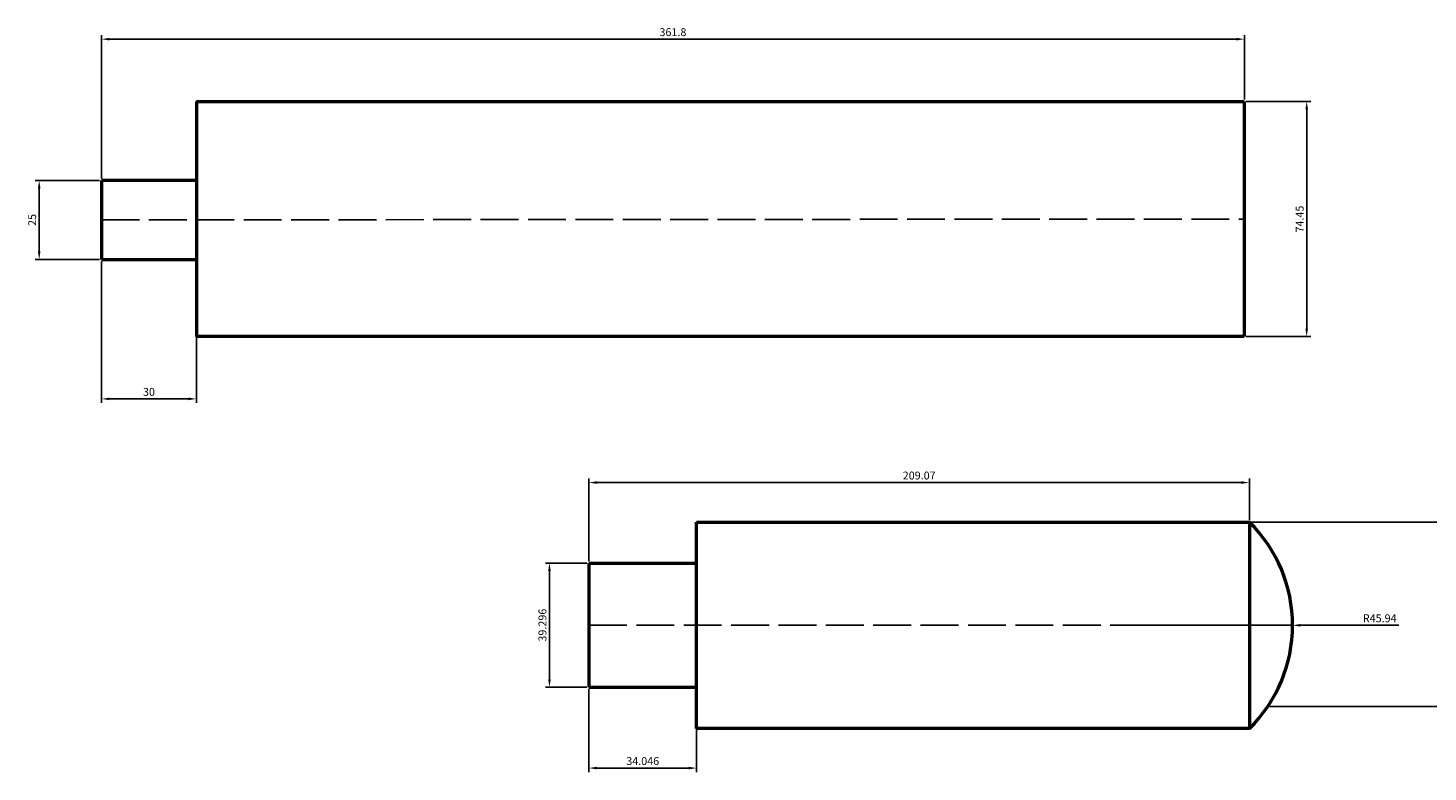
# Model space of a CAD drawing. Units: millimetres. Extents: x 921 to 2648, y 1390 to 2315.
# Tile 6 of 10: x 1762 to 2205, y 1390 to 1625. Entities that reach past the tile are written whole.
import ezdxf

# ---------------------------------------------------------------- set-up
doc = ezdxf.new("R2010")
doc.units = ezdxf.units.MM
doc.linetypes.add('ACAD_ISO02W100', pattern=[15, 12, -3])
for name, color, linetype, lineweight in [('M-DIMS', 2, 'Continuous', 25), ('M-HIDN', 4, 'ACAD_ISO02W100', 25), ('M-OUTL', 7, 'Continuous', 50)]:
    doc.layers.add(name, color=color, linetype=linetype, lineweight=lineweight)
doc.styles.get("Standard").update_dxf_attribs({"font": 'arial.ttf'})
doc.dimstyles.new('ISO-25', dxfattribs={"dimtxt": 2.5, "dimasz": 2.5, "dimexe": 1.25, "dimexo": 0.625, "dimtad": 1, "dimtxsty": 'Standard', "dimcen": 2.5, "dimadec": 0, "dimazin": 0, "dimtfac": 1, "dimtmove": 0, "dimatfit": 3, "dimfxl": 1, "dimarcsym": 0})

# ---------------------------------------------------------------- blocks, each defined once
blk = doc.blocks.new('*D37')
at = {"layer": 'Defpoints', "color": 0, "transparency": 16777216}
for p in [(2146.72, 1621.94), (2146.72, 1602.19), (1784.95, 1577.19)]:
    blk.add_point(p, dxfattribs=at)
at = {"layer": 'M-DIMS', "color": 0, "lineweight": -2, "transparency": 16777216}
for p, q in [((1784.95, 1577.82), (1784.95, 1623.19)), ((2146.72, 1602.82), (2146.72, 1623.19)), ((1787.45, 1621.94), (2144.22, 1621.94))]:
    blk.add_line(p, q, dxfattribs=at)
at = {"layer": 'M-DIMS', "color": 0, "transparency": 16777216}
for points in [[(1787.45, 1622.36), (1787.45, 1621.53), (1784.95, 1621.94)], [(2144.22, 1622.36), (2144.22, 1621.53), (2146.72, 1621.94)]]:
    blk.add_solid(points, dxfattribs=at)
at = {"layer": 'M-DIMS', "color": 0, "transparency": 16777216, "insert": (1965.83, 1623.85), "char_height": 2.5, "attachment_point": 5}
blk.add_mtext('361.8', dxfattribs=at)
blk = doc.blocks.new('*D38')
at = {"layer": 'Defpoints', "color": 0, "transparency": 16777216}
for p in [(2146.72, 1602.19), (2146.72, 1527.75), (2166.47, 1527.75)]:
    blk.add_point(p, dxfattribs=at)
at = {"layer": 'M-DIMS', "color": 0, "lineweight": -2, "transparency": 16777216}
for p, q in [((2147.34, 1602.19), (2167.72, 1602.19)), ((2166.47, 1599.69), (2166.47, 1530.25)), ((2147.34, 1527.75), (2167.72, 1527.75))]:
    blk.add_line(p, q, dxfattribs=at)
at = {"layer": 'M-DIMS', "color": 0, "transparency": 16777216}
for points in [[(2166.05, 1599.69), (2166.88, 1599.69), (2166.47, 1602.19)], [(2166.05, 1530.25), (2166.88, 1530.25), (2166.47, 1527.75)]]:
    blk.add_solid(points, dxfattribs=at)
at = {"layer": 'M-DIMS', "color": 0, "transparency": 16777216, "insert": (2164.57, 1564.97), "char_height": 2.5, "attachment_point": 5, "rotation": 90}
blk.add_mtext('74.45', dxfattribs=at)
blk = doc.blocks.new('*D39')
at = {"layer": 'Defpoints', "color": 0, "transparency": 16777216}
for p in [(2148.31, 1481.5), (2148.31, 1469), (1939.24, 1455.99)]:
    blk.add_point(p, dxfattribs=at)
at = {"layer": 'M-DIMS', "color": 0, "lineweight": -2, "transparency": 16777216}
for p, q in [((1939.24, 1456.61), (1939.24, 1482.75)), ((1941.74, 1481.5), (2145.81, 1481.5)), ((2148.31, 1469.62), (2148.31, 1482.75))]:
    blk.add_line(p, q, dxfattribs=at)
at = {"layer": 'M-DIMS', "color": 0, "transparency": 16777216}
for points in [[(1941.74, 1481.91), (1941.74, 1481.08), (1939.24, 1481.5)], [(2145.81, 1481.91), (2145.81, 1481.08), (2148.31, 1481.5)]]:
    blk.add_solid(points, dxfattribs=at)
at = {"layer": 'M-DIMS', "color": 0, "transparency": 16777216, "insert": (2043.78, 1483.4), "char_height": 2.5, "attachment_point": 5}
blk.add_mtext('209.07', dxfattribs=at)
blk = doc.blocks.new('*D40')
at = {"layer": 'Defpoints', "color": 0, "transparency": 16777216}
for p in [(2148.31, 1469), (2154.14, 1410.59), (2646.82, 1410.59)]:
    blk.add_point(p, dxfattribs=at)
at = {"layer": 'M-DIMS', "color": 0, "lineweight": -2, "transparency": 16777216}
for p, q in [((2148.94, 1469), (2648.07, 1469)), ((2646.82, 1466.5), (2646.82, 1413.09)), ((2154.77, 1410.59), (2648.07, 1410.59))]:
    blk.add_line(p, q, dxfattribs=at)
at = {"layer": 'M-DIMS', "color": 0, "transparency": 16777216}
for points in [[(2646.41, 1466.5), (2647.24, 1466.5), (2646.82, 1469)], [(2646.41, 1413.09), (2647.24, 1413.09), (2646.82, 1410.59)]]:
    blk.add_solid(points, dxfattribs=at)
at = {"layer": 'M-DIMS', "color": 0, "transparency": 16777216, "insert": (2644.92, 1439.79), "char_height": 2.5, "attachment_point": 5, "rotation": 90}
blk.add_mtext('58.41', dxfattribs=at)
blk = doc.blocks.new('*D98')
at = {"layer": 'Defpoints', "color": 0, "transparency": 16777216}
for p in [(1784.95, 1552.19), (1814.95, 1552.19), (1814.95, 1508)]:
    blk.add_point(p, dxfattribs=at)
at = {"layer": 'M-DIMS', "color": 0, "lineweight": -2, "transparency": 16777216}
for p, q in [((1784.95, 1551.57), (1784.95, 1506.75)), ((1814.95, 1551.57), (1814.95, 1506.75)), ((1787.45, 1508), (1812.45, 1508))]:
    blk.add_line(p, q, dxfattribs=at)
at = {"layer": 'M-DIMS', "color": 0, "transparency": 16777216}
for points in [[(1787.45, 1508.41), (1787.45, 1507.58), (1784.95, 1508)], [(1812.45, 1508.41), (1812.45, 1507.58), (1814.95, 1508)]]:
    blk.add_solid(points, dxfattribs=at)
at = {"layer": 'M-DIMS', "color": 0, "transparency": 16777216, "insert": (1799.95, 1509.9), "char_height": 2.5, "attachment_point": 5}
blk.add_mtext('30', dxfattribs=at)
blk = doc.blocks.new('*D99')
at = {"layer": 'Defpoints', "color": 0, "transparency": 16777216}
for p in [(1784.95, 1577.19), (1765.2, 1552.19), (1784.95, 1552.19)]:
    blk.add_point(p, dxfattribs=at)
at = {"layer": 'M-DIMS', "color": 0, "lineweight": -2, "transparency": 16777216}
for p, q in [((1784.32, 1577.19), (1763.95, 1577.19)), ((1765.2, 1574.69), (1765.2, 1554.69)), ((1784.32, 1552.19), (1763.95, 1552.19))]:
    blk.add_line(p, q, dxfattribs=at)
at = {"layer": 'M-DIMS', "color": 0, "transparency": 16777216}
for points in [[(1764.78, 1574.69), (1765.61, 1574.69), (1765.2, 1577.19)], [(1764.78, 1554.69), (1765.61, 1554.69), (1765.2, 1552.19)]]:
    blk.add_solid(points, dxfattribs=at)
at = {"layer": 'M-DIMS', "color": 0, "transparency": 16777216, "insert": (1763.3, 1564.69), "char_height": 2.5, "attachment_point": 5, "rotation": 90}
blk.add_mtext('25', dxfattribs=at)
blk = doc.blocks.new('*D100')
at = {"layer": 'Defpoints', "color": 0, "transparency": 16777216}
for p in [(1939.24, 1416.69), (1973.29, 1416.69), (1973.29, 1391.06)]:
    blk.add_point(p, dxfattribs=at)
at = {"layer": 'M-DIMS', "color": 0, "lineweight": -2, "transparency": 16777216}
for p, q in [((1939.24, 1416.07), (1939.24, 1389.81)), ((1973.29, 1416.07), (1973.29, 1389.81)), ((1941.74, 1391.06), (1970.79, 1391.06))]:
    blk.add_line(p, q, dxfattribs=at)
at = {"layer": 'M-DIMS', "color": 0, "transparency": 16777216}
for points in [[(1941.74, 1391.48), (1941.74, 1390.65), (1939.24, 1391.06)], [(1970.79, 1391.48), (1970.79, 1390.65), (1973.29, 1391.06)]]:
    blk.add_solid(points, dxfattribs=at)
at = {"layer": 'M-DIMS', "color": 0, "transparency": 16777216, "insert": (1956.26, 1392.96), "char_height": 2.5, "attachment_point": 5}
blk.add_mtext('34.046', dxfattribs=at)
blk = doc.blocks.new('*D101')
at = {"layer": 'Defpoints', "color": 0, "transparency": 16777216}
for p in [(1939.24, 1455.99), (1926.74, 1416.69), (1939.24, 1416.69)]:
    blk.add_point(p, dxfattribs=at)
at = {"layer": 'M-DIMS', "color": 0, "lineweight": -2, "transparency": 16777216}
for p, q in [((1938.62, 1455.99), (1925.49, 1455.99)), ((1926.74, 1453.49), (1926.74, 1419.19)), ((1938.62, 1416.69), (1925.49, 1416.69))]:
    blk.add_line(p, q, dxfattribs=at)
at = {"layer": 'M-DIMS', "color": 0, "transparency": 16777216}
for points in [[(1926.32, 1453.49), (1927.16, 1453.49), (1926.74, 1455.99)], [(1926.32, 1419.19), (1927.16, 1419.19), (1926.74, 1416.69)]]:
    blk.add_solid(points, dxfattribs=at)
at = {"layer": 'M-DIMS', "color": 0, "transparency": 16777216, "insert": (1924.84, 1436.34), "char_height": 2.5, "attachment_point": 5, "rotation": 90}
blk.add_mtext('39.296', dxfattribs=at)
blk = doc.blocks.new('*D122')
at = {"layer": 'Defpoints', "color": 0, "transparency": 16777216}
for p in [(2116.06, 1436.28), (2162, 1436.28)]:
    blk.add_point(p, dxfattribs=at)
at = {"layer": 'M-DIMS', "color": 0, "lineweight": -2, "transparency": 16777216}
for p, q in [((2116.06, 1436.28), (2162, 1436.28)), ((2195.6, 1436.28), (2164.5, 1436.28))]:
    blk.add_line(p, q, dxfattribs=at)
at = {"layer": 'M-DIMS', "color": 0, "transparency": 16777216}
blk.add_solid([(2164.5, 1436.7), (2164.5, 1435.86), (2162, 1436.28)], dxfattribs=at)
at = {"layer": 'M-DIMS', "color": 0, "transparency": 16777216, "insert": (2189.57, 1438.18), "char_height": 2.5, "attachment_point": 5, "rotation": 359.9996}
blk.add_mtext('R45.94', dxfattribs=at)

msp = doc.modelspace()

# ---------------------------------------------------------------- linework, layer by layer
at = {"layer": 'M-HIDN'}
for p, q in [((1784.9467, 1564.6949), (2146.7158, 1564.97)), ((1939.2411, 1436.3404), (2161.9999, 1436.2803))]:
    msp.add_line(p, q, dxfattribs=at)
at = {"layer": 'M-OUTL'}
for p, q in [((1814.9467, 1602.1949), (2146.7158, 1602.1949)), ((1814.9467, 1602.1949), (1814.9467, 1527.7451)), ((1814.9467, 1602.1949), (1814.9467, 1577.1949)), ((2146.7158, 1602.1949), (2146.7158, 1527.7451)), ((1814.9467, 1577.1949), (1784.9467, 1577.1949)), ((1784.9467, 1577.1949), (1784.9467, 1552.1949)), ((1784.9467, 1552.1949), (1814.9467, 1552.1949)), ((2146.7158, 1527.7451), (1814.9467, 1527.7451)), ((1973.2872, 1468.998), (2148.3108, 1468.998)), ((1973.2872, 1403.5626), (1973.2872, 1468.998)), ((2148.3108, 1468.998), (2148.3108, 1403.5626)), ((1939.2411, 1455.9884), (1973.2872, 1455.9884)), ((1939.2411, 1455.9884), (1939.2411, 1416.6925)), ((1939.2411, 1416.6925), (1973.2872, 1416.6925)), ((2148.3108, 1403.5626), (1973.2872, 1403.5626))]:
    msp.add_line(p, q, dxfattribs=at)
msp.add_arc((2116.057, 1436.2803), 45.943, 314.590918, 45.409082, dxfattribs=at)

# ---------------------------------------------------------------- dimensions: what is measured, and where the dimension line sits
at = {"layer": 'M-DIMS'}
for base, p1, p2, override, picture, middle in [((2146.7158, 1621.9449), (1784.9467, 1577.1949), (2146.7158, 1602.1949), {"dimdec": 1, "dimlfac": 1, "dimrnd": 0, "dimzin": 0, "dimdsep": 46, "dimlunit": 2}, '*D37', (1965.8312, 1623.8471)), ((1814.9467, 1507.9951), (1784.9467, 1552.1949), (1814.9467, 1552.1949), {"dimdec": 0, "dimlfac": 1, "dimrnd": 0, "dimzin": 0, "dimdsep": 46, "dimlunit": 2}, '*D98', (1799.9467, 1509.8973)), ((2148.3108, 1481.498), (1939.2411, 1455.9884), (2148.3108, 1468.998), {"dimdec": 2, "dimlfac": 1, "dimrnd": 0, "dimzin": 0, "dimdsep": 46, "dimlunit": 2}, '*D39', (2043.7759, 1483.3994)), ((1973.2872, 1391.0626), (1939.2411, 1416.6925), (1973.2872, 1416.6925), {"dimdec": 3, "dimlfac": 1, "dimrnd": 0, "dimzin": 0, "dimdsep": 46, "dimlunit": 2}, '*D100', (1956.2641, 1392.9649))]:
    dim = msp.add_linear_dim(base=base, p1=p1, p2=p2, dimstyle='ISO-25', override=override, dxfattribs=at)
    dim.commit()
    dim.dimension.update_dxf_attribs({"geometry": picture, "text_midpoint": middle})
for base, p1, p2, override, picture, middle in [((2166.4658, 1527.7451), (2146.7158, 1602.1949), (2146.7158, 1527.7451), {"dimdec": 2, "dimlfac": 1, "dimrnd": 0, "dimzin": 0, "dimdsep": 46, "dimlunit": 2}, '*D38', (2164.5695, 1564.97)), ((1765.1967, 1552.1949), (1784.9467, 1577.1949), (1784.9467, 1552.1949), {"dimdec": 0, "dimlfac": 1, "dimrnd": 0, "dimzin": 0, "dimdsep": 46, "dimlunit": 2}, '*D99', (1763.2952, 1564.6949)), ((2646.8247, 1410.5877), (2148.3108, 1468.998), (2154.1446, 1410.5877), {"dimdec": 2, "dimlfac": 1, "dimrnd": 0, "dimzin": 0, "dimdsep": 46, "dimlunit": 2}, '*D40', (2644.9233, 1439.7929)), ((1926.7411, 1416.6925), (1939.2411, 1455.9884), (1939.2411, 1416.6925), {"dimdec": 3, "dimlfac": 1, "dimrnd": 0, "dimzin": 0, "dimdsep": 46, "dimlunit": 2}, '*D101', (1924.8388, 1436.3404))]:
    dim = msp.add_linear_dim(base=base, p1=p1, p2=p2, angle=90, dimstyle='ISO-25', override=override, dxfattribs=at)
    dim.commit()
    dim.dimension.update_dxf_attribs({"geometry": picture, "text_midpoint": middle})
dim = msp.add_radius_dim(center=(2116.057, 1436.2803), mpoint=(2161.9999, 1436.28), dimstyle='ISO-25', override={"dimdec": 2, "dimlfac": 1, "dimrnd": 0, "dimzin": 0, "dimdsep": 46, "dimlunit": 2}, dxfattribs=at)
dim.commit()
dim.dimension.update_dxf_attribs({"geometry": '*D122', "text_midpoint": (2189.5657, 1436.2798), "dimtype": 164})

doc.saveas('drawing.dxf')
